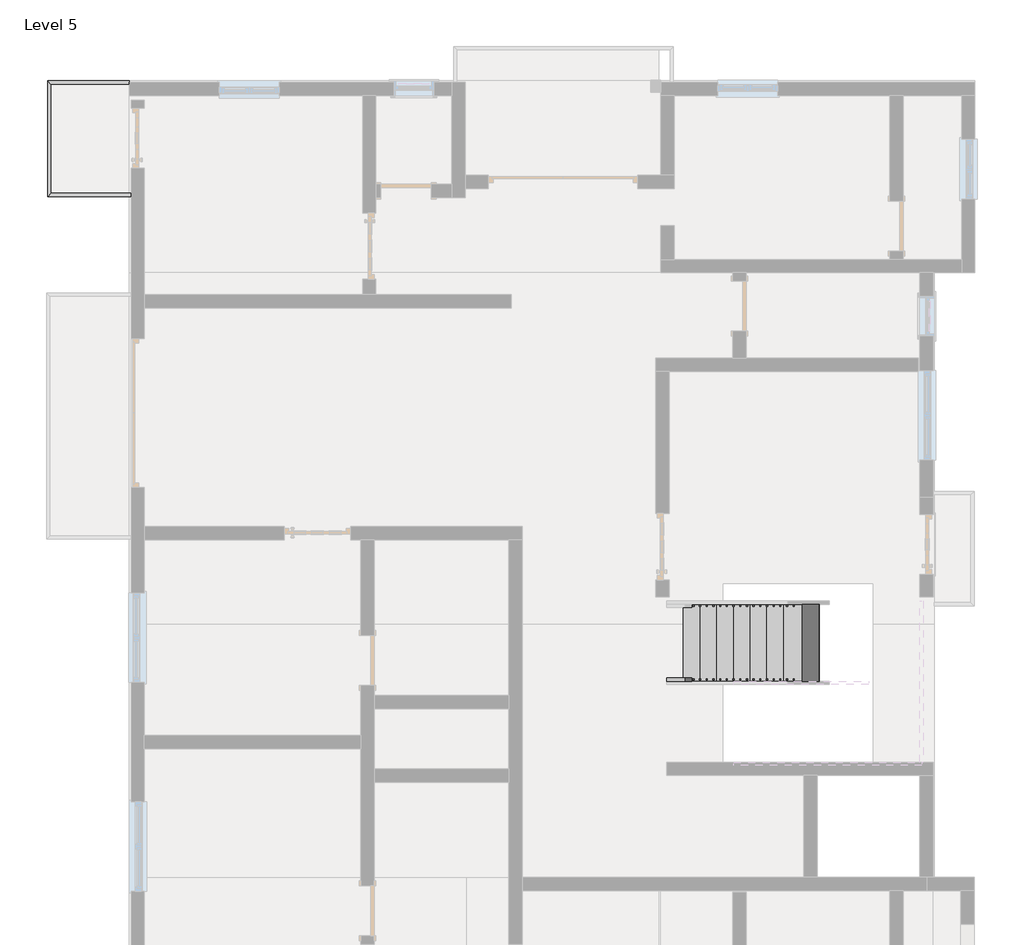
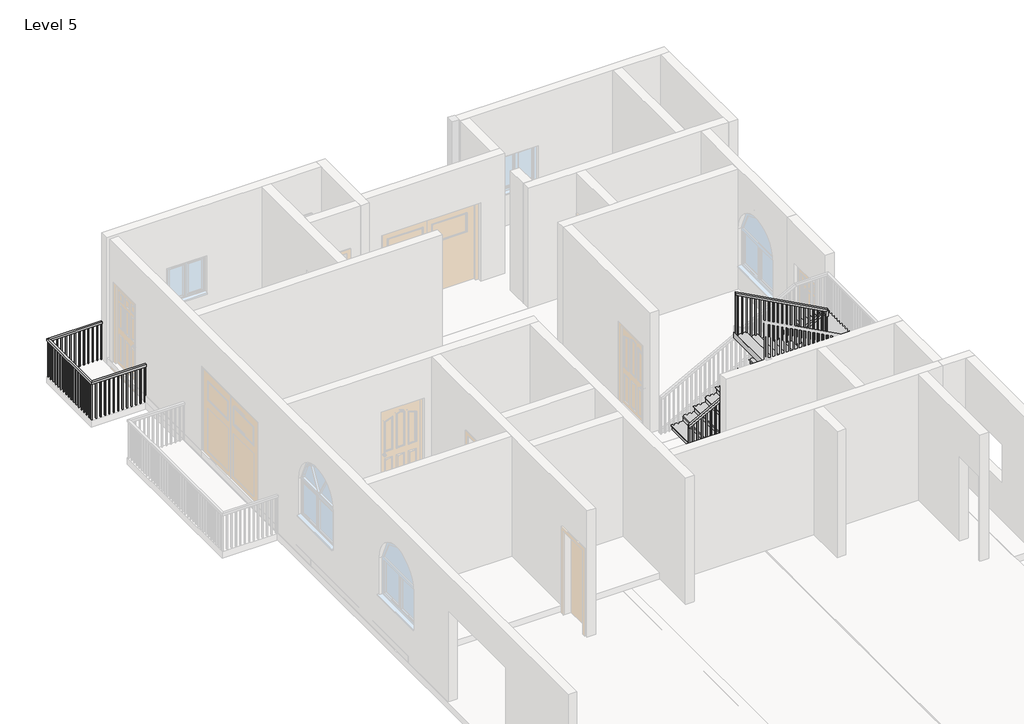
# One storey, part 5 of 7: 2 railings, 1 stair flight.
"""IFC4 building model written with IfcOpenShell, lengths in millimetres."""

from ifc_helpers import new_model, si_unit, frame, origin, place, context, project, spatial, polyline, outline, extrude, faceted_brep, transform, mapped, element, save
from components import stair_flight_7472872d

model = new_model("IFC4")

# Units and contexts
model_context = context("Model", 3, world=origin())
ifc_project = project(units=[si_unit("LENGTHUNIT", "METRE", prefix="MILLI")], contexts=[model_context])

# Site, building, storey
site = spatial("IfcSite", under=ifc_project)
building = spatial("IfcBuilding", under=site)
storey = spatial("IfcBuildingStorey", under=building, Name="Level 5", Elevation=12192.0)

# Railings
placement = place(None, origin())
element("IfcRailing", 1, ObjectType="Handrail - Rectangular", at=placement, inside=storey, context=model_context, shape_type="SolidModel", body=[
    faceted_brep([(-6354.2109037, 9376.4527313, 13106.4), (-6354.2109037, 9376.4527313, 13055.6), (-6354.2109037, 9427.2527313, 13055.6), (-6354.2109037, 9427.2527313, 13106.4), (-7548.0109037, 9376.4527313, 13106.4), (-7548.0109037, 9376.4527313, 13055.6), (-7598.8109037, 9427.2527313, 13055.6), (-7598.8109037, 9427.2527313, 13106.4), (-7548.0109037, 7717.9584215, 13106.4), (-7548.0109037, 7717.9584215, 13055.6), (-7598.8109037, 7667.1584215, 13055.6), (-7598.8109037, 7667.1584215, 13106.4), (-6330.8013636, 7717.9584215, 13106.4), (-6330.8013636, 7667.1584215, 13106.4), (-6330.8013636, 7667.1584215, 13055.6), (-6330.8013636, 7717.9584215, 13055.6)], [[[0, 1, 2, 3]], [[1, 0, 4, 5]], [[2, 1, 5, 6]], [[3, 2, 6, 7]], [[0, 3, 7, 4]], [[5, 4, 8, 9]], [[6, 5, 9, 10]], [[7, 6, 10, 11]], [[4, 7, 11, 8]], [[12, 13, 14, 15]], [[9, 8, 12, 15]], [[10, 9, 15, 14]], [[11, 10, 14, 13]], [[8, 11, 13, 12]]]),
    extrude(outline(polyline([(-6363.7359037, 7683.0334215), (-6363.7359037, 7702.0834215), (-6344.6859037, 7702.0834215), (-6344.6859037, 7683.0334215), (-6363.7359037, 7683.0334215)])), frame((0.0, 0.0, 12192.0), z_axis=(0.0, 0.0, 1.0), x_axis=(1.0, 0.0, 0.0)), (0.0, 0.0, 1.0), 863.6),
    extrude(outline(polyline([(-6465.3359037, 7683.0334215), (-6465.3359037, 7702.0834215), (-6446.2859037, 7702.0834215), (-6446.2859037, 7683.0334215), (-6465.3359037, 7683.0334215)])), frame((0.0, 0.0, 12192.0), z_axis=(0.0, 0.0, 1.0), x_axis=(1.0, 0.0, 0.0)), (0.0, 0.0, 1.0), 863.6),
    extrude(outline(polyline([(-6566.9359037, 7683.0334215), (-6566.9359037, 7702.0834215), (-6547.8859037, 7702.0834215), (-6547.8859037, 7683.0334215), (-6566.9359037, 7683.0334215)])), frame((0.0, 0.0, 12192.0), z_axis=(0.0, 0.0, 1.0), x_axis=(1.0, 0.0, 0.0)), (0.0, 0.0, 1.0), 863.6),
    extrude(outline(polyline([(-6668.5359037, 7683.0334215), (-6668.5359037, 7702.0834215), (-6649.4859037, 7702.0834215), (-6649.4859037, 7683.0334215), (-6668.5359037, 7683.0334215)])), frame((0.0, 0.0, 12192.0), z_axis=(0.0, 0.0, 1.0), x_axis=(1.0, 0.0, 0.0)), (0.0, 0.0, 1.0), 863.6),
    extrude(outline(polyline([(-6770.1359037, 7683.0334215), (-6770.1359037, 7702.0834215), (-6751.0859037, 7702.0834215), (-6751.0859037, 7683.0334215), (-6770.1359037, 7683.0334215)])), frame((0.0, 0.0, 12192.0), z_axis=(0.0, 0.0, 1.0), x_axis=(1.0, 0.0, 0.0)), (0.0, 0.0, 1.0), 863.6),
    extrude(outline(polyline([(-6871.7359037, 7683.0334215), (-6871.7359037, 7702.0834215), (-6852.6859037, 7702.0834215), (-6852.6859037, 7683.0334215), (-6871.7359037, 7683.0334215)])), frame((0.0, 0.0, 12192.0), z_axis=(0.0, 0.0, 1.0), x_axis=(1.0, 0.0, 0.0)), (0.0, 0.0, 1.0), 863.6),
    extrude(outline(polyline([(-6973.3359037, 7683.0334215), (-6973.3359037, 7702.0834215), (-6954.2859037, 7702.0834215), (-6954.2859037, 7683.0334215), (-6973.3359037, 7683.0334215)])), frame((0.0, 0.0, 12192.0), z_axis=(0.0, 0.0, 1.0), x_axis=(1.0, 0.0, 0.0)), (0.0, 0.0, 1.0), 863.6),
    extrude(outline(polyline([(-7074.9359037, 7683.0334215), (-7074.9359037, 7702.0834215), (-7055.8859037, 7702.0834215), (-7055.8859037, 7683.0334215), (-7074.9359037, 7683.0334215)])), frame((0.0, 0.0, 12192.0), z_axis=(0.0, 0.0, 1.0), x_axis=(1.0, 0.0, 0.0)), (0.0, 0.0, 1.0), 863.6),
    extrude(outline(polyline([(-7176.5359037, 7683.0334215), (-7176.5359037, 7702.0834215), (-7157.4859037, 7702.0834215), (-7157.4859037, 7683.0334215), (-7176.5359037, 7683.0334215)])), frame((0.0, 0.0, 12192.0), z_axis=(0.0, 0.0, 1.0), x_axis=(1.0, 0.0, 0.0)), (0.0, 0.0, 1.0), 863.6),
    extrude(outline(polyline([(-7278.1359037, 7683.0334215), (-7278.1359037, 7702.0834215), (-7259.0859037, 7702.0834215), (-7259.0859037, 7683.0334215), (-7278.1359037, 7683.0334215)])), frame((0.0, 0.0, 12192.0), z_axis=(0.0, 0.0, 1.0), x_axis=(1.0, 0.0, 0.0)), (0.0, 0.0, 1.0), 863.6),
    extrude(outline(polyline([(-7379.7359037, 7683.0334215), (-7379.7359037, 7702.0834215), (-7360.6859037, 7702.0834215), (-7360.6859037, 7683.0334215), (-7379.7359037, 7683.0334215)])), frame((0.0, 0.0, 12192.0), z_axis=(0.0, 0.0, 1.0), x_axis=(1.0, 0.0, 0.0)), (0.0, 0.0, 1.0), 863.6),
    extrude(outline(polyline([(-7481.3359037, 7683.0334215), (-7481.3359037, 7702.0834215), (-7462.2859037, 7702.0834215), (-7462.2859037, 7683.0334215), (-7481.3359037, 7683.0334215)])), frame((0.0, 0.0, 12192.0), z_axis=(0.0, 0.0, 1.0), x_axis=(1.0, 0.0, 0.0)), (0.0, 0.0, 1.0), 863.6),
    extrude(outline(polyline([(-7582.9359037, 7785.7777313), (-7563.8859037, 7785.7777313), (-7563.8859037, 7766.7277313), (-7582.9359037, 7766.7277313), (-7582.9359037, 7785.7777313)])), frame((0.0, 0.0, 12192.0), z_axis=(0.0, 0.0, 1.0), x_axis=(1.0, 0.0, 0.0)), (0.0, 0.0, 1.0), 863.6),
    extrude(outline(polyline([(-7582.9359037, 7887.3777313), (-7563.8859037, 7887.3777313), (-7563.8859037, 7868.3277313), (-7582.9359037, 7868.3277313), (-7582.9359037, 7887.3777313)])), frame((0.0, 0.0, 12192.0), z_axis=(0.0, 0.0, 1.0), x_axis=(1.0, 0.0, 0.0)), (0.0, 0.0, 1.0), 863.6),
    extrude(outline(polyline([(-7582.9359037, 7988.9777313), (-7563.8859037, 7988.9777313), (-7563.8859037, 7969.9277313), (-7582.9359037, 7969.9277313), (-7582.9359037, 7988.9777313)])), frame((0.0, 0.0, 12192.0), z_axis=(0.0, 0.0, 1.0), x_axis=(1.0, 0.0, 0.0)), (0.0, 0.0, 1.0), 863.6),
    extrude(outline(polyline([(-7582.9359037, 8090.5777313), (-7563.8859037, 8090.5777313), (-7563.8859037, 8071.5277313), (-7582.9359037, 8071.5277313), (-7582.9359037, 8090.5777313)])), frame((0.0, 0.0, 12192.0), z_axis=(0.0, 0.0, 1.0), x_axis=(1.0, 0.0, 0.0)), (0.0, 0.0, 1.0), 863.6),
    extrude(outline(polyline([(-7582.9359037, 8192.1777313), (-7563.8859037, 8192.1777313), (-7563.8859037, 8173.1277313), (-7582.9359037, 8173.1277313), (-7582.9359037, 8192.1777313)])), frame((0.0, 0.0, 12192.0), z_axis=(0.0, 0.0, 1.0), x_axis=(1.0, 0.0, 0.0)), (0.0, 0.0, 1.0), 863.6),
    extrude(outline(polyline([(-7582.9359037, 8293.7777313), (-7563.8859037, 8293.7777313), (-7563.8859037, 8274.7277313), (-7582.9359037, 8274.7277313), (-7582.9359037, 8293.7777313)])), frame((0.0, 0.0, 12192.0), z_axis=(0.0, 0.0, 1.0), x_axis=(1.0, 0.0, 0.0)), (0.0, 0.0, 1.0), 863.6),
    extrude(outline(polyline([(-7582.9359037, 8395.3777313), (-7563.8859037, 8395.3777313), (-7563.8859037, 8376.3277313), (-7582.9359037, 8376.3277313), (-7582.9359037, 8395.3777313)])), frame((0.0, 0.0, 12192.0), z_axis=(0.0, 0.0, 1.0), x_axis=(1.0, 0.0, 0.0)), (0.0, 0.0, 1.0), 863.6),
    extrude(outline(polyline([(-7582.9359037, 8496.9777313), (-7563.8859037, 8496.9777313), (-7563.8859037, 8477.9277313), (-7582.9359037, 8477.9277313), (-7582.9359037, 8496.9777313)])), frame((0.0, 0.0, 12192.0), z_axis=(0.0, 0.0, 1.0), x_axis=(1.0, 0.0, 0.0)), (0.0, 0.0, 1.0), 863.6),
    extrude(outline(polyline([(-7582.9359037, 8598.5777313), (-7563.8859037, 8598.5777313), (-7563.8859037, 8579.5277313), (-7582.9359037, 8579.5277313), (-7582.9359037, 8598.5777313)])), frame((0.0, 0.0, 12192.0), z_axis=(0.0, 0.0, 1.0), x_axis=(1.0, 0.0, 0.0)), (0.0, 0.0, 1.0), 863.6),
    extrude(outline(polyline([(-7582.9359037, 8700.1777313), (-7563.8859037, 8700.1777313), (-7563.8859037, 8681.1277313), (-7582.9359037, 8681.1277313), (-7582.9359037, 8700.1777313)])), frame((0.0, 0.0, 12192.0), z_axis=(0.0, 0.0, 1.0), x_axis=(1.0, 0.0, 0.0)), (0.0, 0.0, 1.0), 863.6),
    extrude(outline(polyline([(-7582.9359037, 8801.7777313), (-7563.8859037, 8801.7777313), (-7563.8859037, 8782.7277313), (-7582.9359037, 8782.7277313), (-7582.9359037, 8801.7777313)])), frame((0.0, 0.0, 12192.0), z_axis=(0.0, 0.0, 1.0), x_axis=(1.0, 0.0, 0.0)), (0.0, 0.0, 1.0), 863.6),
    extrude(outline(polyline([(-7582.9359037, 8903.3777313), (-7563.8859037, 8903.3777313), (-7563.8859037, 8884.3277313), (-7582.9359037, 8884.3277313), (-7582.9359037, 8903.3777313)])), frame((0.0, 0.0, 12192.0), z_axis=(0.0, 0.0, 1.0), x_axis=(1.0, 0.0, 0.0)), (0.0, 0.0, 1.0), 863.6),
    extrude(outline(polyline([(-7582.9359037, 9004.9777313), (-7563.8859037, 9004.9777313), (-7563.8859037, 8985.9277313), (-7582.9359037, 8985.9277313), (-7582.9359037, 9004.9777313)])), frame((0.0, 0.0, 12192.0), z_axis=(0.0, 0.0, 1.0), x_axis=(1.0, 0.0, 0.0)), (0.0, 0.0, 1.0), 863.6),
    extrude(outline(polyline([(-7582.9359037, 9106.5777313), (-7563.8859037, 9106.5777313), (-7563.8859037, 9087.5277313), (-7582.9359037, 9087.5277313), (-7582.9359037, 9106.5777313)])), frame((0.0, 0.0, 12192.0), z_axis=(0.0, 0.0, 1.0), x_axis=(1.0, 0.0, 0.0)), (0.0, 0.0, 1.0), 863.6),
    extrude(outline(polyline([(-7582.9359037, 9208.1777313), (-7563.8859037, 9208.1777313), (-7563.8859037, 9189.1277313), (-7582.9359037, 9189.1277313), (-7582.9359037, 9208.1777313)])), frame((0.0, 0.0, 12192.0), z_axis=(0.0, 0.0, 1.0), x_axis=(1.0, 0.0, 0.0)), (0.0, 0.0, 1.0), 863.6),
    extrude(outline(polyline([(-7582.9359037, 9309.7777313), (-7563.8859037, 9309.7777313), (-7563.8859037, 9290.7277313), (-7582.9359037, 9290.7277313), (-7582.9359037, 9309.7777313)])), frame((0.0, 0.0, 12192.0), z_axis=(0.0, 0.0, 1.0), x_axis=(1.0, 0.0, 0.0)), (0.0, 0.0, 1.0), 863.6),
    extrude(outline(polyline([(-7462.2859037, 9411.3777313), (-7462.2859037, 9392.3277313), (-7481.3359037, 9392.3277313), (-7481.3359037, 9411.3777313), (-7462.2859037, 9411.3777313)])), frame((0.0, 0.0, 12192.0), z_axis=(0.0, 0.0, 1.0), x_axis=(1.0, 0.0, 0.0)), (0.0, 0.0, 1.0), 863.6),
    extrude(outline(polyline([(-7360.6859037, 9411.3777313), (-7360.6859037, 9392.3277313), (-7379.7359037, 9392.3277313), (-7379.7359037, 9411.3777313), (-7360.6859037, 9411.3777313)])), frame((0.0, 0.0, 12192.0), z_axis=(0.0, 0.0, 1.0), x_axis=(1.0, 0.0, 0.0)), (0.0, 0.0, 1.0), 863.6),
    extrude(outline(polyline([(-7259.0859037, 9411.3777313), (-7259.0859037, 9392.3277313), (-7278.1359037, 9392.3277313), (-7278.1359037, 9411.3777313), (-7259.0859037, 9411.3777313)])), frame((0.0, 0.0, 12192.0), z_axis=(0.0, 0.0, 1.0), x_axis=(1.0, 0.0, 0.0)), (0.0, 0.0, 1.0), 863.6),
    extrude(outline(polyline([(-7157.4859037, 9411.3777313), (-7157.4859037, 9392.3277313), (-7176.5359037, 9392.3277313), (-7176.5359037, 9411.3777313), (-7157.4859037, 9411.3777313)])), frame((0.0, 0.0, 12192.0), z_axis=(0.0, 0.0, 1.0), x_axis=(1.0, 0.0, 0.0)), (0.0, 0.0, 1.0), 863.6),
    extrude(outline(polyline([(-7055.8859037, 9411.3777313), (-7055.8859037, 9392.3277313), (-7074.9359037, 9392.3277313), (-7074.9359037, 9411.3777313), (-7055.8859037, 9411.3777313)])), frame((0.0, 0.0, 12192.0), z_axis=(0.0, 0.0, 1.0), x_axis=(1.0, 0.0, 0.0)), (0.0, 0.0, 1.0), 863.6),
    extrude(outline(polyline([(-6954.2859037, 9411.3777313), (-6954.2859037, 9392.3277313), (-6973.3359037, 9392.3277313), (-6973.3359037, 9411.3777313), (-6954.2859037, 9411.3777313)])), frame((0.0, 0.0, 12192.0), z_axis=(0.0, 0.0, 1.0), x_axis=(1.0, 0.0, 0.0)), (0.0, 0.0, 1.0), 863.6),
    extrude(outline(polyline([(-6852.6859037, 9411.3777313), (-6852.6859037, 9392.3277313), (-6871.7359037, 9392.3277313), (-6871.7359037, 9411.3777313), (-6852.6859037, 9411.3777313)])), frame((0.0, 0.0, 12192.0), z_axis=(0.0, 0.0, 1.0), x_axis=(1.0, 0.0, 0.0)), (0.0, 0.0, 1.0), 863.6),
    extrude(outline(polyline([(-6751.0859037, 9411.3777313), (-6751.0859037, 9392.3277313), (-6770.1359037, 9392.3277313), (-6770.1359037, 9411.3777313), (-6751.0859037, 9411.3777313)])), frame((0.0, 0.0, 12192.0), z_axis=(0.0, 0.0, 1.0), x_axis=(1.0, 0.0, 0.0)), (0.0, 0.0, 1.0), 863.6),
    extrude(outline(polyline([(-6649.4859037, 9411.3777313), (-6649.4859037, 9392.3277313), (-6668.5359037, 9392.3277313), (-6668.5359037, 9411.3777313), (-6649.4859037, 9411.3777313)])), frame((0.0, 0.0, 12192.0), z_axis=(0.0, 0.0, 1.0), x_axis=(1.0, 0.0, 0.0)), (0.0, 0.0, 1.0), 863.6),
    extrude(outline(polyline([(-6547.8859037, 9411.3777313), (-6547.8859037, 9392.3277313), (-6566.9359037, 9392.3277313), (-6566.9359037, 9411.3777313), (-6547.8859037, 9411.3777313)])), frame((0.0, 0.0, 12192.0), z_axis=(0.0, 0.0, 1.0), x_axis=(1.0, 0.0, 0.0)), (0.0, 0.0, 1.0), 863.6),
    extrude(outline(polyline([(-6446.2859037, 9411.3777313), (-6446.2859037, 9392.3277313), (-6465.3359037, 9392.3277313), (-6465.3359037, 9411.3777313), (-6446.2859037, 9411.3777313)])), frame((0.0, 0.0, 12192.0), z_axis=(0.0, 0.0, 1.0), x_axis=(1.0, 0.0, 0.0)), (0.0, 0.0, 1.0), 863.6),
    extrude(outline(polyline([(-7582.9359037, 7702.0834215), (-7563.8859037, 7702.0834215), (-7563.8859037, 7683.0334215), (-7582.9359037, 7683.0334215), (-7582.9359037, 7702.0834215)])), frame((0.0, 0.0, 12192.0), z_axis=(0.0, 0.0, 1.0), x_axis=(1.0, 0.0, 0.0)), (0.0, 0.0, 1.0), 863.6),
    extrude(outline(polyline([(-7563.8859037, 9411.3777313), (-7563.8859037, 9392.3277313), (-7582.9359037, 9392.3277313), (-7582.9359037, 9411.3777313), (-7563.8859037, 9411.3777313)])), frame((0.0, 0.0, 12192.0), z_axis=(0.0, 0.0, 1.0), x_axis=(1.0, 0.0, 0.0)), (0.0, 0.0, 1.0), 863.6),
    extrude(outline(polyline([(-6349.8513636, 7683.0334215), (-6349.8513636, 7702.0834215), (-6330.8013636, 7702.0834215), (-6330.8013636, 7683.0334215), (-6349.8513636, 7683.0334215)])), frame((0.0, 0.0, 12192.0), z_axis=(0.0, 0.0, 1.0), x_axis=(1.0, 0.0, 0.0)), (0.0, 0.0, 1.0), 863.6),
    extrude(outline(polyline([(-6354.2109037, 9411.3777313), (-6354.2109037, 9392.3277313), (-6373.2609037, 9392.3277313), (-6373.2609037, 9411.3777313), (-6354.2109037, 9411.3777313)])), frame((0.0, 0.0, 12192.0), z_axis=(0.0, 0.0, 1.0), x_axis=(1.0, 0.0, 0.0)), (0.0, 0.0, 1.0), 863.6),
])
element("IfcRailing", 2, ObjectType="Handrail - Rectangular", at=placement, inside=storey, context=model_context, shape_type="SolidModel", body=[
    faceted_brep([(1811.8890963, 347.1962251, 13244.9454545), (1811.8890963, 347.1962251, 13187.1709673), (1811.8890963, 296.3962251, 13187.1709673), (1811.8890963, 296.3962251, 13244.9454545), (4804.8326586, 347.1962251, 14866.2136078), (4855.6326586, 347.1962251, 14835.9573214), (4855.6326586, 296.3962251, 14835.9573214), (4804.8326586, 296.3962251, 14866.2136078), (4804.8326586, 347.1962251, 14907.4909091), (4855.6326586, 347.1962251, 14856.6909091), (4855.6326586, 296.3962251, 14856.6909091), (4804.8326586, 296.3962251, 14907.4909091), (4931.8326586, 347.1962251, 14907.4909091), (4931.8326586, 347.1962251, 14856.6909091), (4881.0326586, 296.3962251, 14856.6909091), (4881.0326586, 296.3962251, 14907.4909091), (4931.8326586, 245.5962251, 14907.4909091), (4881.0326586, 245.5962251, 14907.4909091), (4881.0326586, 194.7962251, 14856.6909091), (4931.8326586, 194.7962251, 14856.6909091)], [[[0, 1, 2, 3]], [[1, 0, 4, 5]], [[2, 1, 5, 6]], [[3, 2, 6, 7]], [[0, 3, 7, 4]], [[5, 4, 8, 9]], [[6, 5, 9, 10]], [[7, 6, 10, 11]], [[4, 7, 11, 8]], [[9, 8, 12, 13]], [[10, 9, 13, 14]], [[11, 10, 14, 15]], [[8, 11, 15, 12]], [[16, 17, 18, 19]], [[13, 12, 16, 19]], [[14, 13, 19, 18]], [[15, 14, 18, 17]], [[12, 15, 17, 16]]]),
    faceted_brep([(4931.8326586, 245.5962251, 14907.4909091), (4931.8326586, 194.7962251, 14856.6909091), (4881.0326586, 194.7962251, 14856.6909091), (4881.0326586, 245.5962251, 14907.4909091), (4931.8326586, 245.5962251, 15018.6126249), (4881.0326586, 245.5962251, 14988.3068093), (4881.0326586, 194.7962251, 14988.3068093), (4931.8326586, 194.7962251, 15018.6126249)], [[[0, 1, 2, 3]], [[4, 5, 6, 7]], [[1, 0, 4, 7]], [[2, 1, 7, 6]], [[3, 2, 6, 5]], [[0, 3, 5, 4]]]),
    faceted_brep([(4931.8326586, 194.7962251, 15018.6126249), (4881.0326586, 194.7962251, 14988.3068093), (4881.0326586, 245.5962251, 14988.3068093), (4931.8326586, 245.5962251, 15018.6126249), (2827.8890963, 194.7962251, 16154.4), (2827.8890963, 245.5962251, 16154.4), (2827.8890963, 245.5962251, 16096.6704456), (2827.8890963, 194.7962251, 16096.6704456)], [[[0, 1, 2, 3]], [[4, 5, 6, 7]], [[1, 0, 4, 7]], [[2, 1, 7, 6]], [[3, 2, 6, 5]], [[0, 3, 5, 4]]]),
    extrude(outline(polyline([(16066.40254, 2883.9576586), (16076.686442, 2864.9076586), (15101.4545455, 2864.9076586), (15101.4545455, 2883.9576586), (16066.40254, 2883.9576586)])), frame((0.0, 210.6712251, 0.0), z_axis=(0.0, 1.0, 0.0), x_axis=(0.0, 0.0, 1.0)), (0.0, 0.0, 1.0), 19.05),
    extrude(outline(polyline([(16011.5550624, 2985.5576586), (16021.8389645, 2966.5076586), (15101.4545455, 2966.5076586), (15101.4545455, 2985.5576586), (16011.5550624, 2985.5576586)])), frame((0.0, 210.6712251, 0.0), z_axis=(0.0, 1.0, 0.0), x_axis=(0.0, 0.0, 1.0)), (0.0, 0.0, 1.0), 19.05),
    extrude(outline(polyline([(15956.7075849, 3087.1576586), (15966.9914869, 3068.1076586), (15101.4545455, 3068.1076586), (15101.4545455, 3087.1576586), (15956.7075849, 3087.1576586)])), frame((0.0, 210.6712251, 0.0), z_axis=(0.0, 1.0, 0.0), x_axis=(0.0, 0.0, 1.0)), (0.0, 0.0, 1.0), 19.05),
    extrude(outline(polyline([(15901.8601073, 3188.7576586), (15912.1440094, 3169.7076586), (14962.9090909, 3169.7076586), (14962.9090909, 3188.7576586), (15901.8601073, 3188.7576586)])), frame((0.0, 210.6712251, 0.0), z_axis=(0.0, 1.0, 0.0), x_axis=(0.0, 0.0, 1.0)), (0.0, 0.0, 1.0), 19.05),
    extrude(outline(polyline([(15847.0126298, 3290.3576586), (15857.2965318, 3271.3076586), (14962.9090909, 3271.3076586), (14962.9090909, 3290.3576586), (15847.0126298, 3290.3576586)])), frame((0.0, 210.6712251, 0.0), z_axis=(0.0, 1.0, 0.0), x_axis=(0.0, 0.0, 1.0)), (0.0, 0.0, 1.0), 19.05),
    extrude(outline(polyline([(15792.1651522, 3391.9576586), (15802.4490542, 3372.9076586), (14824.3636364, 3372.9076586), (14824.3636364, 3391.9576586), (15792.1651522, 3391.9576586)])), frame((0.0, 210.6712251, 0.0), z_axis=(0.0, 1.0, 0.0), x_axis=(0.0, 0.0, 1.0)), (0.0, 0.0, 1.0), 19.05),
    extrude(outline(polyline([(15737.3176746, 3493.5576586), (15747.6015767, 3474.5076586), (14824.3636364, 3474.5076586), (14824.3636364, 3493.5576586), (15737.3176746, 3493.5576586)])), frame((0.0, 210.6712251, 0.0), z_axis=(0.0, 1.0, 0.0), x_axis=(0.0, 0.0, 1.0)), (0.0, 0.0, 1.0), 19.05),
    extrude(outline(polyline([(15682.4701971, 3595.1576586), (15692.7540991, 3576.1076586), (14824.3636364, 3576.1076586), (14824.3636364, 3595.1576586), (15682.4701971, 3595.1576586)])), frame((0.0, 210.6712251, 0.0), z_axis=(0.0, 1.0, 0.0), x_axis=(0.0, 0.0, 1.0)), (0.0, 0.0, 1.0), 19.05),
    extrude(outline(polyline([(15627.6227195, 3696.7576586), (15637.9066216, 3677.7076586), (14685.8181818, 3677.7076586), (14685.8181818, 3696.7576586), (15627.6227195, 3696.7576586)])), frame((0.0, 210.6712251, 0.0), z_axis=(0.0, 1.0, 0.0), x_axis=(0.0, 0.0, 1.0)), (0.0, 0.0, 1.0), 19.05),
    extrude(outline(polyline([(15572.775242, 3798.3576586), (15583.059144, 3779.3076586), (14685.8181818, 3779.3076586), (14685.8181818, 3798.3576586), (15572.775242, 3798.3576586)])), frame((0.0, 210.6712251, 0.0), z_axis=(0.0, 1.0, 0.0), x_axis=(0.0, 0.0, 1.0)), (0.0, 0.0, 1.0), 19.05),
    extrude(outline(polyline([(15517.9277644, 3899.9576586), (15528.2116665, 3880.9076586), (14547.2727273, 3880.9076586), (14547.2727273, 3899.9576586), (15517.9277644, 3899.9576586)])), frame((0.0, 210.6712251, 0.0), z_axis=(0.0, 1.0, 0.0), x_axis=(0.0, 0.0, 1.0)), (0.0, 0.0, 1.0), 19.05),
    extrude(outline(polyline([(15463.0802869, 4001.5576586), (15473.3641889, 3982.5076586), (14547.2727273, 3982.5076586), (14547.2727273, 4001.5576586), (15463.0802869, 4001.5576586)])), frame((0.0, 210.6712251, 0.0), z_axis=(0.0, 1.0, 0.0), x_axis=(0.0, 0.0, 1.0)), (0.0, 0.0, 1.0), 19.05),
    extrude(outline(polyline([(15408.2328093, 4103.1576586), (15418.5167113, 4084.1076586), (14547.2727273, 4084.1076586), (14547.2727273, 4103.1576586), (15408.2328093, 4103.1576586)])), frame((0.0, 210.6712251, 0.0), z_axis=(0.0, 1.0, 0.0), x_axis=(0.0, 0.0, 1.0)), (0.0, 0.0, 1.0), 19.05),
    extrude(outline(polyline([(15353.3853317, 4204.7576586), (15363.6692338, 4185.7076586), (14408.7272727, 4185.7076586), (14408.7272727, 4204.7576586), (15353.3853317, 4204.7576586)])), frame((0.0, 210.6712251, 0.0), z_axis=(0.0, 1.0, 0.0), x_axis=(0.0, 0.0, 1.0)), (0.0, 0.0, 1.0), 19.05),
    extrude(outline(polyline([(15298.5378542, 4306.3576586), (15308.8217562, 4287.3076586), (14408.7272727, 4287.3076586), (14408.7272727, 4306.3576586), (15298.5378542, 4306.3576586)])), frame((0.0, 210.6712251, 0.0), z_axis=(0.0, 1.0, 0.0), x_axis=(0.0, 0.0, 1.0)), (0.0, 0.0, 1.0), 19.05),
    extrude(outline(polyline([(15243.6903766, 4407.9576586), (15253.9742787, 4388.9076586), (14270.1818182, 4388.9076586), (14270.1818182, 4407.9576586), (15243.6903766, 4407.9576586)])), frame((0.0, 210.6712251, 0.0), z_axis=(0.0, 1.0, 0.0), x_axis=(0.0, 0.0, 1.0)), (0.0, 0.0, 1.0), 19.05),
    extrude(outline(polyline([(15188.8428991, 4509.5576586), (15199.1268011, 4490.5076586), (14270.1818182, 4490.5076586), (14270.1818182, 4509.5576586), (15188.8428991, 4509.5576586)])), frame((0.0, 210.6712251, 0.0), z_axis=(0.0, 1.0, 0.0), x_axis=(0.0, 0.0, 1.0)), (0.0, 0.0, 1.0), 19.05),
    extrude(outline(polyline([(15133.9954215, 4611.1576586), (15144.2793236, 4592.1076586), (14270.1818182, 4592.1076586), (14270.1818182, 4611.1576586), (15133.9954215, 4611.1576586)])), frame((0.0, 210.6712251, 0.0), z_axis=(0.0, 1.0, 0.0), x_axis=(0.0, 0.0, 1.0)), (0.0, 0.0, 1.0), 19.05),
    extrude(outline(polyline([(15079.147944, 4712.7576586), (15089.431846, 4693.7076586), (14131.6363636, 4693.7076586), (14131.6363636, 4712.7576586), (15079.147944, 4712.7576586)])), frame((0.0, 210.6712251, 0.0), z_axis=(0.0, 1.0, 0.0), x_axis=(0.0, 0.0, 1.0)), (0.0, 0.0, 1.0), 19.05),
    extrude(outline(polyline([(15024.3004664, 4814.3576586), (15034.5843684, 4795.3076586), (14131.6363636, 4795.3076586), (14131.6363636, 4814.3576586), (15024.3004664, 4814.3576586)])), frame((0.0, 210.6712251, 0.0), z_axis=(0.0, 1.0, 0.0), x_axis=(0.0, 0.0, 1.0)), (0.0, 0.0, 1.0), 19.05),
    extrude(outline(polyline([(4850.3640963, 312.2712251), (4850.3640963, 331.3212251), (4869.4140963, 331.3212251), (4869.4140963, 312.2712251), (4850.3640963, 312.2712251)])), frame((0.0, 0.0, 13854.5454545), z_axis=(0.0, 0.0, 1.0), x_axis=(1.0, 0.0, 0.0)), (0.0, 0.0, 1.0), 1002.1454545),
    extrude(outline(polyline([(14788.3862812, 4767.8140963), (14778.0669559, 4748.7640963), (13854.5454545, 4748.7640963), (13854.5454545, 4767.8140963), (14788.3862812, 4767.8140963)])), frame((0.0, 312.2712251, 0.0), z_axis=(0.0, 1.0, 0.0), x_axis=(0.0, 0.0, 1.0)), (0.0, 0.0, 1.0), 19.05),
    extrude(outline(polyline([(14733.3498795, 4666.2140963), (14723.0305541, 4647.1640963), (13854.5454545, 4647.1640963), (13854.5454545, 4666.2140963), (14733.3498795, 4666.2140963)])), frame((0.0, 312.2712251, 0.0), z_axis=(0.0, 1.0, 0.0), x_axis=(0.0, 0.0, 1.0)), (0.0, 0.0, 1.0), 19.05),
    extrude(outline(polyline([(14678.3134777, 4564.6140963), (14667.9941524, 4545.5640963), (13716.0, 4545.5640963), (13716.0, 4564.6140963), (14678.3134777, 4564.6140963)])), frame((0.0, 312.2712251, 0.0), z_axis=(0.0, 1.0, 0.0), x_axis=(0.0, 0.0, 1.0)), (0.0, 0.0, 1.0), 19.05),
    extrude(outline(polyline([(14623.2770759, 4463.0140963), (14612.9577506, 4443.9640963), (13716.0, 4443.9640963), (13716.0, 4463.0140963), (14623.2770759, 4463.0140963)])), frame((0.0, 312.2712251, 0.0), z_axis=(0.0, 1.0, 0.0), x_axis=(0.0, 0.0, 1.0)), (0.0, 0.0, 1.0), 19.05),
    extrude(outline(polyline([(14568.2406742, 4361.4140963), (14557.9213488, 4342.3640963), (13716.0, 4342.3640963), (13716.0, 4361.4140963), (14568.2406742, 4361.4140963)])), frame((0.0, 312.2712251, 0.0), z_axis=(0.0, 1.0, 0.0), x_axis=(0.0, 0.0, 1.0)), (0.0, 0.0, 1.0), 19.05),
    extrude(outline(polyline([(14513.2042724, 4259.8140963), (14502.8849471, 4240.7640963), (13577.4545455, 4240.7640963), (13577.4545455, 4259.8140963), (14513.2042724, 4259.8140963)])), frame((0.0, 312.2712251, 0.0), z_axis=(0.0, 1.0, 0.0), x_axis=(0.0, 0.0, 1.0)), (0.0, 0.0, 1.0), 19.05),
    extrude(outline(polyline([(14458.1678706, 4158.2140963), (14447.8485453, 4139.1640963), (13577.4545455, 4139.1640963), (13577.4545455, 4158.2140963), (14458.1678706, 4158.2140963)])), frame((0.0, 312.2712251, 0.0), z_axis=(0.0, 1.0, 0.0), x_axis=(0.0, 0.0, 1.0)), (0.0, 0.0, 1.0), 19.05),
    extrude(outline(polyline([(14403.1314688, 4056.6140963), (14392.8121435, 4037.5640963), (13438.9090909, 4037.5640963), (13438.9090909, 4056.6140963), (14403.1314688, 4056.6140963)])), frame((0.0, 312.2712251, 0.0), z_axis=(0.0, 1.0, 0.0), x_axis=(0.0, 0.0, 1.0)), (0.0, 0.0, 1.0), 19.05),
    extrude(outline(polyline([(14348.0950671, 3955.0140963), (14337.7757417, 3935.9640963), (13438.9090909, 3935.9640963), (13438.9090909, 3955.0140963), (14348.0950671, 3955.0140963)])), frame((0.0, 312.2712251, 0.0), z_axis=(0.0, 1.0, 0.0), x_axis=(0.0, 0.0, 1.0)), (0.0, 0.0, 1.0), 19.05),
    extrude(outline(polyline([(14293.0586653, 3853.4140963), (14282.73934, 3834.3640963), (13438.9090909, 3834.3640963), (13438.9090909, 3853.4140963), (14293.0586653, 3853.4140963)])), frame((0.0, 312.2712251, 0.0), z_axis=(0.0, 1.0, 0.0), x_axis=(0.0, 0.0, 1.0)), (0.0, 0.0, 1.0), 19.05),
    extrude(outline(polyline([(14238.0222635, 3751.8140963), (14227.7029382, 3732.7640963), (13300.3636364, 3732.7640963), (13300.3636364, 3751.8140963), (14238.0222635, 3751.8140963)])), frame((0.0, 312.2712251, 0.0), z_axis=(0.0, 1.0, 0.0), x_axis=(0.0, 0.0, 1.0)), (0.0, 0.0, 1.0), 19.05),
    extrude(outline(polyline([(14182.9858618, 3650.2140963), (14172.6665364, 3631.1640963), (13300.3636364, 3631.1640963), (13300.3636364, 3650.2140963), (14182.9858618, 3650.2140963)])), frame((0.0, 312.2712251, 0.0), z_axis=(0.0, 1.0, 0.0), x_axis=(0.0, 0.0, 1.0)), (0.0, 0.0, 1.0), 19.05),
    extrude(outline(polyline([(14127.94946, 3548.6140963), (14117.6301347, 3529.5640963), (13161.8181818, 3529.5640963), (13161.8181818, 3548.6140963), (14127.94946, 3548.6140963)])), frame((0.0, 312.2712251, 0.0), z_axis=(0.0, 1.0, 0.0), x_axis=(0.0, 0.0, 1.0)), (0.0, 0.0, 1.0), 19.05),
    extrude(outline(polyline([(14072.9130582, 3447.0140963), (14062.5937329, 3427.9640963), (13161.8181818, 3427.9640963), (13161.8181818, 3447.0140963), (14072.9130582, 3447.0140963)])), frame((0.0, 312.2712251, 0.0), z_axis=(0.0, 1.0, 0.0), x_axis=(0.0, 0.0, 1.0)), (0.0, 0.0, 1.0), 19.05),
    extrude(outline(polyline([(14017.8766565, 3345.4140963), (14007.5573311, 3326.3640963), (13161.8181818, 3326.3640963), (13161.8181818, 3345.4140963), (14017.8766565, 3345.4140963)])), frame((0.0, 312.2712251, 0.0), z_axis=(0.0, 1.0, 0.0), x_axis=(0.0, 0.0, 1.0)), (0.0, 0.0, 1.0), 19.05),
    extrude(outline(polyline([(13962.8402547, 3243.8140963), (13952.5209294, 3224.7640963), (13023.2727273, 3224.7640963), (13023.2727273, 3243.8140963), (13962.8402547, 3243.8140963)])), frame((0.0, 312.2712251, 0.0), z_axis=(0.0, 1.0, 0.0), x_axis=(0.0, 0.0, 1.0)), (0.0, 0.0, 1.0), 19.05),
    extrude(outline(polyline([(13907.8038529, 3142.2140963), (13897.4845276, 3123.1640963), (13023.2727273, 3123.1640963), (13023.2727273, 3142.2140963), (13907.8038529, 3142.2140963)])), frame((0.0, 312.2712251, 0.0), z_axis=(0.0, 1.0, 0.0), x_axis=(0.0, 0.0, 1.0)), (0.0, 0.0, 1.0), 19.05),
    extrude(outline(polyline([(13852.7674512, 3040.6140963), (13842.4481258, 3021.5640963), (12884.7272727, 3021.5640963), (12884.7272727, 3040.6140963), (13852.7674512, 3040.6140963)])), frame((0.0, 312.2712251, 0.0), z_axis=(0.0, 1.0, 0.0), x_axis=(0.0, 0.0, 1.0)), (0.0, 0.0, 1.0), 19.05),
    extrude(outline(polyline([(13797.7310494, 2939.0140963), (13787.4117241, 2919.9640963), (12884.7272727, 2919.9640963), (12884.7272727, 2939.0140963), (13797.7310494, 2939.0140963)])), frame((0.0, 312.2712251, 0.0), z_axis=(0.0, 1.0, 0.0), x_axis=(0.0, 0.0, 1.0)), (0.0, 0.0, 1.0), 19.05),
    extrude(outline(polyline([(13742.6946476, 2837.4140963), (13732.3753223, 2818.3640963), (12884.7272727, 2818.3640963), (12884.7272727, 2837.4140963), (13742.6946476, 2837.4140963)])), frame((0.0, 312.2712251, 0.0), z_axis=(0.0, 1.0, 0.0), x_axis=(0.0, 0.0, 1.0)), (0.0, 0.0, 1.0), 19.05),
    extrude(outline(polyline([(13687.6582459, 2735.8140963), (13677.3389205, 2716.7640963), (12746.1818182, 2716.7640963), (12746.1818182, 2735.8140963), (13687.6582459, 2735.8140963)])), frame((0.0, 312.2712251, 0.0), z_axis=(0.0, 1.0, 0.0), x_axis=(0.0, 0.0, 1.0)), (0.0, 0.0, 1.0), 19.05),
    extrude(outline(polyline([(13632.6218441, 2634.2140963), (13622.3025188, 2615.1640963), (12746.1818182, 2615.1640963), (12746.1818182, 2634.2140963), (13632.6218441, 2634.2140963)])), frame((0.0, 312.2712251, 0.0), z_axis=(0.0, 1.0, 0.0), x_axis=(0.0, 0.0, 1.0)), (0.0, 0.0, 1.0), 19.05),
    extrude(outline(polyline([(13577.5854423, 2532.6140963), (13567.266117, 2513.5640963), (12607.6363636, 2513.5640963), (12607.6363636, 2532.6140963), (13577.5854423, 2532.6140963)])), frame((0.0, 312.2712251, 0.0), z_axis=(0.0, 1.0, 0.0), x_axis=(0.0, 0.0, 1.0)), (0.0, 0.0, 1.0), 19.05),
    extrude(outline(polyline([(13522.5490405, 2431.0140963), (13512.2297152, 2411.9640963), (12607.6363636, 2411.9640963), (12607.6363636, 2431.0140963), (13522.5490405, 2431.0140963)])), frame((0.0, 312.2712251, 0.0), z_axis=(0.0, 1.0, 0.0), x_axis=(0.0, 0.0, 1.0)), (0.0, 0.0, 1.0), 19.05),
    extrude(outline(polyline([(13467.5126388, 2329.4140963), (13457.1933134, 2310.3640963), (12607.6363636, 2310.3640963), (12607.6363636, 2329.4140963), (13467.5126388, 2329.4140963)])), frame((0.0, 312.2712251, 0.0), z_axis=(0.0, 1.0, 0.0), x_axis=(0.0, 0.0, 1.0)), (0.0, 0.0, 1.0), 19.05),
    extrude(outline(polyline([(13412.476237, 2227.8140963), (13402.1569117, 2208.7640963), (12469.0909091, 2208.7640963), (12469.0909091, 2227.8140963), (13412.476237, 2227.8140963)])), frame((0.0, 312.2712251, 0.0), z_axis=(0.0, 1.0, 0.0), x_axis=(0.0, 0.0, 1.0)), (0.0, 0.0, 1.0), 19.05),
    extrude(outline(polyline([(13357.4398352, 2126.2140963), (13347.1205099, 2107.1640963), (12469.0909091, 2107.1640963), (12469.0909091, 2126.2140963), (13357.4398352, 2126.2140963)])), frame((0.0, 312.2712251, 0.0), z_axis=(0.0, 1.0, 0.0), x_axis=(0.0, 0.0, 1.0)), (0.0, 0.0, 1.0), 19.05),
    extrude(outline(polyline([(13302.4034335, 2024.6140963), (13292.0841081, 2005.5640963), (12330.5454545, 2005.5640963), (12330.5454545, 2024.6140963), (13302.4034335, 2024.6140963)])), frame((0.0, 312.2712251, 0.0), z_axis=(0.0, 1.0, 0.0), x_axis=(0.0, 0.0, 1.0)), (0.0, 0.0, 1.0), 19.05),
    extrude(outline(polyline([(13247.3670317, 1923.0140963), (13237.0477064, 1903.9640963), (12330.5454545, 1903.9640963), (12330.5454545, 1923.0140963), (13247.3670317, 1923.0140963)])), frame((0.0, 312.2712251, 0.0), z_axis=(0.0, 1.0, 0.0), x_axis=(0.0, 0.0, 1.0)), (0.0, 0.0, 1.0), 19.05),
    extrude(outline(polyline([(4896.9076586, 229.7212251), (4915.9576586, 229.7212251), (4915.9576586, 210.6712251), (4896.9076586, 210.6712251), (4896.9076586, 229.7212251)])), frame((0.0, 0.0, 13993.0909091), z_axis=(0.0, 0.0, 1.0), x_axis=(1.0, 0.0, 0.0)), (0.0, 0.0, 1.0), 863.6),
    extrude(outline(polyline([(4896.9076586, 312.2712251), (4896.9076586, 331.3212251), (4915.9576586, 331.3212251), (4915.9576586, 312.2712251), (4896.9076586, 312.2712251)])), frame((0.0, 0.0, 13993.0909091), z_axis=(0.0, 0.0, 1.0), x_axis=(1.0, 0.0, 0.0)), (0.0, 0.0, 1.0), 863.6),
    extrude(outline(polyline([(16086.3865436, 2846.9390963), (16096.6704456, 2827.8890963), (15101.4545455, 2827.8890963), (15101.4545455, 2846.9390963), (16086.3865436, 2846.9390963)])), frame((0.0, 210.6712251, 0.0), z_axis=(0.0, 1.0, 0.0), x_axis=(0.0, 0.0, 1.0)), (0.0, 0.0, 1.0), 19.05),
    extrude(outline(polyline([(13197.4902926, 1830.9390963), (13187.1709673, 1811.8890963), (12330.5454545, 1811.8890963), (12330.5454545, 1830.9390963), (13197.4902926, 1830.9390963)])), frame((0.0, 312.2712251, 0.0), z_axis=(0.0, 1.0, 0.0), x_axis=(0.0, 0.0, 1.0)), (0.0, 0.0, 1.0), 19.05),
])

# Stair flight
stair_flight_shape = stair_flight_7472872d(model_context)
element("IfcStairFlight", 3, ObjectType="2\" Tread 1\" Nosing 1/4\" Riser", at=placement, inside=storey, context=model_context, shape_type="MappedRepresentation", body=[
    mapped(stair_flight_shape, transform((0.0, 0.0, 0.0), x_axis=(1.0, 0.0, 0.0), y_axis=(0.0, 1.0, 0.0), z_axis=(0.0, 0.0, 1.0))),
])

save(model, "model.ifc")

# Revit data of these elements
# Type "Handrail - Rectangular"
#   Assembly Code = "C2010400"
#   built-in parameter 1008612 = 0.0416667 (stored number, unit not read)
#   built-in parameter 1008611 = 0.0416667 (stored number, unit not read)
#   built-in parameter 1008609 = 0.333333 (stored number, unit not read)
#   built-in parameter 1008604 = 0.166667 (stored number, unit not read)
#   built-in parameter 1008603 = 0.166667 (stored number, unit not read)
#   Railing Height = 3' - 0"
#   built-in parameter 1008630 = 2
#   built-in parameter 1008610 = 2
#   built-in parameter 1008618 = Baluster - Square : 3/4"
# Elements 1, 2 (IfcRailing, "Handrail - Rectangular")
#   Phase Created = New Construction
# Element 3 (IfcStairFlight, "2\" Tread 1\" Nosing 1/4\" Riser")
#   Phase Created = New Construction
